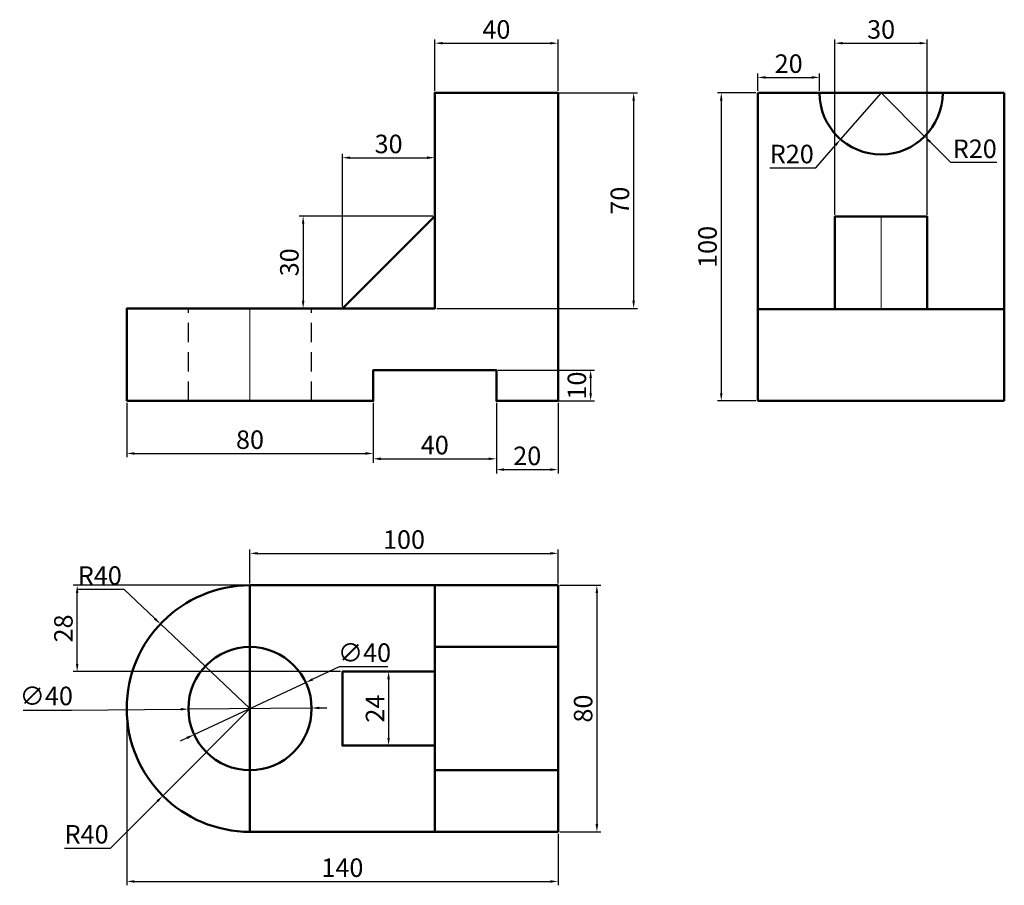
# Model space of a CAD drawing. Units: millimetres. Extents: x 40 to 360, y 50 to 331.
import ezdxf

# ---------------------------------------------------------------- set-up
doc = ezdxf.new("R2010")
doc.units = ezdxf.units.MM
doc.linetypes.add('CENTER', pattern=[50.8, 31.75, -6.35, 6.35, -6.35])
doc.linetypes.add('HIDDEN', pattern=[9.525, 6.35, -3.175])
for name, color, linetype, lineweight in [('M-CNTR', 4, 'CENTER', 18), ('M-DIMS', 2, 'Continuous', 25), ('M-HIDN', 3, 'HIDDEN', 25), ('M-OUTL', 7, 'Continuous', 50)]:
    doc.layers.add(name, color=color, linetype=linetype, lineweight=lineweight)
doc.styles.get("Standard").update_dxf_attribs({"font": 'arial.ttf'})
doc.dimstyles.new('ISO-25', dxfattribs={"dimtxt": 6, "dimasz": 2.5, "dimexe": 1.25, "dimexo": 0.625, "dimtad": 1, "dimtoh": 1, "dimdec": 0, "dimtxsty": 'Standard', "dimcen": 2.5, "dimadec": 0, "dimazin": 0, "dimtfac": 1, "dimtdec": 0, "dimtmove": 0, "dimatfit": 3, "dimfxl": 1, "dimarcsym": 0})

# ---------------------------------------------------------------- blocks, each defined once
blk = doc.blocks.new('*D1')
at = {"layer": 'Defpoints', "color": 0, "transparency": 16777216}
for p in [(74.87, 207.67), (154.87, 207.67), (154.87, 190.64)]:
    blk.add_point(p, dxfattribs=at)
at = {"layer": 'M-DIMS', "color": 0, "lineweight": -2, "transparency": 16777216}
for p, q in [((74.87, 207.05), (74.87, 189.39)), ((154.87, 207.05), (154.87, 189.39)), ((77.37, 190.64), (152.37, 190.64))]:
    blk.add_line(p, q, dxfattribs=at)
at = {"layer": 'M-DIMS', "color": 0, "transparency": 16777216}
for points in [[(77.37, 191.06), (77.37, 190.22), (74.87, 190.64)], [(152.37, 191.06), (152.37, 190.22), (154.87, 190.64)]]:
    blk.add_solid(points, dxfattribs=at)
at = {"layer": 'M-DIMS', "color": 0, "transparency": 16777216, "insert": (114.87, 194.33), "char_height": 6, "attachment_point": 5}
blk.add_mtext('80', dxfattribs=at)
blk = doc.blocks.new('*D2')
at = {"layer": 'Defpoints', "color": 0, "transparency": 16777216}
for p in [(154.87, 207.67), (194.87, 207.67), (194.87, 188.89)]:
    blk.add_point(p, dxfattribs=at)
at = {"layer": 'M-DIMS', "color": 0, "lineweight": -2, "transparency": 16777216}
for p, q in [((154.87, 207.05), (154.87, 187.64)), ((194.87, 207.05), (194.87, 187.64)), ((157.37, 188.89), (192.37, 188.89))]:
    blk.add_line(p, q, dxfattribs=at)
at = {"layer": 'M-DIMS', "color": 0, "transparency": 16777216}
for points in [[(157.37, 189.31), (157.37, 188.47), (154.87, 188.89)], [(192.37, 189.31), (192.37, 188.47), (194.87, 188.89)]]:
    blk.add_solid(points, dxfattribs=at)
at = {"layer": 'M-DIMS', "color": 0, "transparency": 16777216, "insert": (174.87, 192.58), "char_height": 6, "attachment_point": 5}
blk.add_mtext('40', dxfattribs=at)
blk = doc.blocks.new('*D3')
at = {"layer": 'Defpoints', "color": 0, "transparency": 16777216}
for p in [(194.87, 207.67), (214.87, 207.67), (214.87, 185.39)]:
    blk.add_point(p, dxfattribs=at)
at = {"layer": 'M-DIMS', "color": 0, "lineweight": -2, "transparency": 16777216}
for p, q in [((194.87, 207.05), (194.87, 184.14)), ((214.87, 207.05), (214.87, 184.14)), ((197.37, 185.39), (212.37, 185.39))]:
    blk.add_line(p, q, dxfattribs=at)
at = {"layer": 'M-DIMS', "color": 0, "transparency": 16777216}
for points in [[(197.37, 185.81), (197.37, 184.98), (194.87, 185.39)], [(212.37, 185.81), (212.37, 184.98), (214.87, 185.39)]]:
    blk.add_solid(points, dxfattribs=at)
at = {"layer": 'M-DIMS', "color": 0, "transparency": 16777216, "insert": (204.87, 189.08), "char_height": 6, "attachment_point": 5}
blk.add_mtext('20', dxfattribs=at)
blk = doc.blocks.new('*D4')
at = {"layer": 'Defpoints', "color": 0, "transparency": 16777216}
for p in [(174.87, 267.67), (132.12, 237.67), (174.87, 237.67)]:
    blk.add_point(p, dxfattribs=at)
at = {"layer": 'M-DIMS', "color": 0, "lineweight": -2, "transparency": 16777216}
for p, q in [((174.24, 267.67), (130.87, 267.67)), ((132.12, 265.17), (132.12, 240.17)), ((174.24, 237.67), (130.87, 237.67))]:
    blk.add_line(p, q, dxfattribs=at)
at = {"layer": 'M-DIMS', "color": 0, "transparency": 16777216}
for points in [[(131.71, 265.17), (132.54, 265.17), (132.12, 267.67)], [(131.71, 240.17), (132.54, 240.17), (132.12, 237.67)]]:
    blk.add_solid(points, dxfattribs=at)
at = {"layer": 'M-DIMS', "color": 0, "transparency": 16777216, "insert": (128.43, 252.67), "char_height": 6, "attachment_point": 5, "rotation": 90}
blk.add_mtext('30', dxfattribs=at)
blk = doc.blocks.new('*D5')
at = {"layer": 'Defpoints', "color": 0, "transparency": 16777216}
for p in [(174.87, 286.61), (144.87, 237.67), (174.87, 237.67)]:
    blk.add_point(p, dxfattribs=at)
at = {"layer": 'M-DIMS', "color": 0, "lineweight": -2, "transparency": 16777216}
for p, q in [((144.87, 238.3), (144.87, 287.86)), ((174.87, 238.3), (174.87, 287.86)), ((147.37, 286.61), (172.37, 286.61))]:
    blk.add_line(p, q, dxfattribs=at)
at = {"layer": 'M-DIMS', "color": 0, "transparency": 16777216}
for points in [[(147.37, 287.03), (147.37, 286.2), (144.87, 286.61)], [(172.37, 287.03), (172.37, 286.2), (174.87, 286.61)]]:
    blk.add_solid(points, dxfattribs=at)
at = {"layer": 'M-DIMS', "color": 0, "transparency": 16777216, "insert": (159.87, 290.3), "char_height": 6, "attachment_point": 5}
blk.add_mtext('30', dxfattribs=at)
blk = doc.blocks.new('*D6')
at = {"layer": 'Defpoints', "color": 0, "transparency": 16777216}
for p in [(174.87, 307.67), (174.87, 237.67), (239.42, 237.67)]:
    blk.add_point(p, dxfattribs=at)
at = {"layer": 'M-DIMS', "color": 0, "lineweight": -2, "transparency": 16777216}
for p, q in [((175.49, 307.67), (240.67, 307.67)), ((239.42, 305.17), (239.42, 240.17)), ((175.49, 237.67), (240.67, 237.67))]:
    blk.add_line(p, q, dxfattribs=at)
at = {"layer": 'M-DIMS', "color": 0, "transparency": 16777216}
for points in [[(239, 305.17), (239.83, 305.17), (239.42, 307.67)], [(239, 240.17), (239.83, 240.17), (239.42, 237.67)]]:
    blk.add_solid(points, dxfattribs=at)
at = {"layer": 'M-DIMS', "color": 0, "transparency": 16777216, "insert": (235.73, 272.67), "char_height": 6, "attachment_point": 5, "rotation": 90}
blk.add_mtext('70', dxfattribs=at)
blk = doc.blocks.new('*D7')
at = {"layer": 'Defpoints', "color": 0, "transparency": 16777216}
for p in [(194.87, 217.67), (194.87, 207.67), (225.46, 207.67)]:
    blk.add_point(p, dxfattribs=at)
at = {"layer": 'M-DIMS', "color": 0, "lineweight": -2, "transparency": 16777216}
for p, q in [((195.49, 217.67), (226.71, 217.67)), ((225.46, 215.17), (225.46, 210.17)), ((195.49, 207.67), (226.71, 207.67))]:
    blk.add_line(p, q, dxfattribs=at)
at = {"layer": 'M-DIMS', "color": 0, "transparency": 16777216}
for points in [[(225.05, 215.17), (225.88, 215.17), (225.46, 217.67)], [(225.05, 210.17), (225.88, 210.17), (225.46, 207.67)]]:
    blk.add_solid(points, dxfattribs=at)
at = {"layer": 'M-DIMS', "color": 0, "transparency": 16777216, "insert": (221.77, 212.67), "char_height": 6, "attachment_point": 5, "rotation": 90}
blk.add_mtext('10', dxfattribs=at)
blk = doc.blocks.new('*D8')
at = {"layer": 'Defpoints', "color": 0, "transparency": 16777216}
for p in [(279.75, 307.67), (267.86, 207.67), (279.75, 207.67)]:
    blk.add_point(p, dxfattribs=at)
at = {"layer": 'M-DIMS', "color": 0, "lineweight": -2, "transparency": 16777216}
for p, q in [((279.13, 307.67), (266.61, 307.67)), ((267.86, 305.17), (267.86, 210.17)), ((279.13, 207.67), (266.61, 207.67))]:
    blk.add_line(p, q, dxfattribs=at)
at = {"layer": 'M-DIMS', "color": 0, "transparency": 16777216}
for points in [[(267.45, 305.17), (268.28, 305.17), (267.86, 307.67)], [(267.45, 210.17), (268.28, 210.17), (267.86, 207.67)]]:
    blk.add_solid(points, dxfattribs=at)
at = {"layer": 'M-DIMS', "color": 0, "transparency": 16777216, "insert": (264.18, 257.67), "char_height": 6, "attachment_point": 5, "rotation": 90}
blk.add_mtext('100', dxfattribs=at)
blk = doc.blocks.new('*D9')
at = {"layer": 'Defpoints', "color": 0, "transparency": 16777216}
for p in [(299.75, 312.67), (279.75, 307.67), (299.75, 307.67)]:
    blk.add_point(p, dxfattribs=at)
at = {"layer": 'M-DIMS', "color": 0, "lineweight": -2, "transparency": 16777216}
for p, q in [((279.75, 308.3), (279.75, 313.92)), ((299.75, 308.3), (299.75, 313.92)), ((282.25, 312.67), (297.25, 312.67))]:
    blk.add_line(p, q, dxfattribs=at)
at = {"layer": 'M-DIMS', "color": 0, "transparency": 16777216}
for points in [[(282.25, 313.09), (282.25, 312.26), (279.75, 312.67)], [(297.25, 313.09), (297.25, 312.26), (299.75, 312.67)]]:
    blk.add_solid(points, dxfattribs=at)
at = {"layer": 'M-DIMS', "color": 0, "transparency": 16777216, "insert": (289.75, 316.36), "char_height": 6, "attachment_point": 5}
blk.add_mtext('20', dxfattribs=at)
blk = doc.blocks.new('*D10')
at = {"layer": 'Defpoints', "color": 0, "transparency": 16777216}
for p in [(319.75, 307.67), (306.61, 292.59)]:
    blk.add_point(p, dxfattribs=at)
at = {"layer": 'M-DIMS', "color": 0, "lineweight": -2, "transparency": 16777216}
for p, q in [((319.75, 307.67), (306.61, 292.59)), ((298.55, 283.34), (304.97, 290.71)), ((283.61, 283.34), (298.55, 283.34))]:
    blk.add_line(p, q, dxfattribs=at)
at = {"layer": 'M-DIMS', "color": 0, "transparency": 16777216}
blk.add_solid([(304.66, 290.98), (305.28, 290.44), (306.61, 292.59)], dxfattribs=at)
at = {"layer": 'M-DIMS', "color": 0, "transparency": 16777216, "insert": (290.76, 287.03), "char_height": 6, "attachment_point": 5}
blk.add_mtext('R20', dxfattribs=at)
blk = doc.blocks.new('*D11')
at = {"layer": 'Defpoints', "color": 0, "transparency": 16777216}
for p in [(159.87, 119.84), (159.87, 95.84), (159.87, 95.84)]:
    blk.add_point(p, dxfattribs=at)
at = {"layer": 'M-DIMS', "color": 0, "lineweight": -2, "transparency": 16777216}
for p, q in [((160.49, 119.84), (161.12, 119.84)), ((159.87, 117.34), (159.87, 98.34)), ((160.49, 95.84), (161.12, 95.84))]:
    blk.add_line(p, q, dxfattribs=at)
at = {"layer": 'M-DIMS', "color": 0, "transparency": 16777216}
for points in [[(159.45, 117.34), (160.28, 117.34), (159.87, 119.84)], [(159.45, 98.34), (160.28, 98.34), (159.87, 95.84)]]:
    blk.add_solid(points, dxfattribs=at)
at = {"layer": 'M-DIMS', "color": 0, "transparency": 16777216, "insert": (156.23, 107.84), "char_height": 6, "attachment_point": 5, "rotation": 90}
blk.add_mtext('24', dxfattribs=at)
blk = doc.blocks.new('*D12')
at = {"layer": 'Defpoints', "color": 0, "transparency": 16777216}
for p in [(94.87, 107.65), (134.86, 108.02)]:
    blk.add_point(p, dxfattribs=at)
at = {"layer": 'M-DIMS', "color": 0, "lineweight": -2, "transparency": 16777216}
for p, q in [((41.19, 107.3), (56.92, 107.3)), ((56.92, 107.3), (92.37, 107.63)), ((134.86, 108.02), (94.87, 107.65)), ((137.36, 108.05), (139.86, 108.07))]:
    blk.add_line(p, q, dxfattribs=at)
at = {"layer": 'M-DIMS', "color": 0, "transparency": 16777216}
for points in [[(92.36, 108.05), (92.37, 107.21), (94.87, 107.65)], [(137.36, 108.46), (137.37, 107.63), (134.86, 108.02)]]:
    blk.add_solid(points, dxfattribs=at)
at = {"layer": 'M-DIMS', "color": 0, "transparency": 16777216, "insert": (48.75, 111.16), "char_height": 6, "attachment_point": 5}
blk.add_mtext('∅40', dxfattribs=at)
blk = doc.blocks.new('*D13')
at = {"layer": 'Defpoints', "color": 0, "transparency": 16777216}
for p in [(85.8, 135.31), (114.87, 107.84)]:
    blk.add_point(p, dxfattribs=at)
at = {"layer": 'M-DIMS', "color": 0, "lineweight": -2, "transparency": 16777216}
for p, q in [((58.97, 146.55), (73.91, 146.55)), ((73.91, 146.55), (83.98, 137.03)), ((114.87, 107.84), (85.8, 135.31))]:
    blk.add_line(p, q, dxfattribs=at)
at = {"layer": 'M-DIMS', "color": 0, "transparency": 16777216}
blk.add_solid([(84.26, 137.34), (83.69, 136.73), (85.8, 135.31)], dxfattribs=at)
at = {"layer": 'M-DIMS', "color": 0, "transparency": 16777216, "insert": (66.12, 150.24), "char_height": 6, "attachment_point": 5}
blk.add_mtext('R40', dxfattribs=at)
blk = doc.blocks.new('*D14')
at = {"layer": 'Defpoints', "color": 0, "transparency": 16777216}
for p in [(214.87, 158.22), (114.87, 147.84), (214.87, 147.84)]:
    blk.add_point(p, dxfattribs=at)
at = {"layer": 'M-DIMS', "color": 0, "lineweight": -2, "transparency": 16777216}
for p, q in [((114.87, 148.46), (114.87, 159.47)), ((117.37, 158.22), (212.37, 158.22)), ((214.87, 148.46), (214.87, 159.47))]:
    blk.add_line(p, q, dxfattribs=at)
at = {"layer": 'M-DIMS', "color": 0, "transparency": 16777216}
for points in [[(117.37, 158.64), (117.37, 157.8), (114.87, 158.22)], [(212.37, 158.64), (212.37, 157.8), (214.87, 158.22)]]:
    blk.add_solid(points, dxfattribs=at)
at = {"layer": 'M-DIMS', "color": 0, "transparency": 16777216, "insert": (164.87, 161.91), "char_height": 6, "attachment_point": 5}
blk.add_mtext('100', dxfattribs=at)
blk = doc.blocks.new('*D15')
at = {"layer": 'Defpoints', "color": 0, "transparency": 16777216}
for p in [(214.87, 147.84), (214.87, 67.84), (227.49, 67.84)]:
    blk.add_point(p, dxfattribs=at)
at = {"layer": 'M-DIMS', "color": 0, "lineweight": -2, "transparency": 16777216}
for p, q in [((215.49, 147.84), (228.74, 147.84)), ((227.49, 145.34), (227.49, 70.34)), ((215.49, 67.84), (228.74, 67.84))]:
    blk.add_line(p, q, dxfattribs=at)
at = {"layer": 'M-DIMS', "color": 0, "transparency": 16777216}
for points in [[(227.07, 145.34), (227.91, 145.34), (227.49, 147.84)], [(227.07, 70.34), (227.91, 70.34), (227.49, 67.84)]]:
    blk.add_solid(points, dxfattribs=at)
at = {"layer": 'M-DIMS', "color": 0, "transparency": 16777216, "insert": (223.8, 107.84), "char_height": 6, "attachment_point": 5, "rotation": 90}
blk.add_mtext('80', dxfattribs=at)
blk = doc.blocks.new('*D16')
at = {"layer": 'Defpoints', "color": 0, "transparency": 16777216}
for p in [(74.87, 107.84), (214.87, 67.84), (214.87, 51.74)]:
    blk.add_point(p, dxfattribs=at)
at = {"layer": 'M-DIMS', "color": 0, "lineweight": -2, "transparency": 16777216}
for p, q in [((74.87, 107.21), (74.87, 50.49)), ((214.87, 67.21), (214.87, 50.49)), ((77.37, 51.74), (212.37, 51.74))]:
    blk.add_line(p, q, dxfattribs=at)
at = {"layer": 'M-DIMS', "color": 0, "transparency": 16777216}
for points in [[(77.37, 52.16), (77.37, 51.32), (74.87, 51.74)], [(212.37, 52.16), (212.37, 51.32), (214.87, 51.74)]]:
    blk.add_solid(points, dxfattribs=at)
at = {"layer": 'M-DIMS', "color": 0, "transparency": 16777216, "insert": (144.87, 55.43), "char_height": 6, "attachment_point": 5}
blk.add_mtext('140', dxfattribs=at)
blk = doc.blocks.new('*D17')
at = {"layer": 'Defpoints', "color": 0, "transparency": 16777216}
for p in [(214.87, 323.77), (174.87, 307.67), (214.87, 307.67)]:
    blk.add_point(p, dxfattribs=at)
at = {"layer": 'M-DIMS', "color": 0, "lineweight": -2, "transparency": 16777216}
for p, q in [((174.87, 308.3), (174.87, 325.02)), ((177.37, 323.77), (212.37, 323.77)), ((214.87, 308.3), (214.87, 325.02))]:
    blk.add_line(p, q, dxfattribs=at)
at = {"layer": 'M-DIMS', "color": 0, "transparency": 16777216}
for points in [[(177.37, 324.19), (177.37, 323.36), (174.87, 323.77)], [(212.37, 324.19), (212.37, 323.36), (214.87, 323.77)]]:
    blk.add_solid(points, dxfattribs=at)
at = {"layer": 'M-DIMS', "color": 0, "transparency": 16777216, "insert": (194.87, 327.46), "char_height": 6, "attachment_point": 5}
blk.add_mtext('40', dxfattribs=at)
blk = doc.blocks.new('*D18')
at = {"layer": 'Defpoints', "color": 0, "transparency": 16777216}
for p in [(58.77, 147.84), (174.87, 147.84), (144.87, 119.84)]:
    blk.add_point(p, dxfattribs=at)
at = {"layer": 'M-DIMS', "color": 0, "lineweight": -2, "transparency": 16777216}
for p, q in [((174.24, 147.84), (57.52, 147.84)), ((58.77, 122.34), (58.77, 145.34)), ((144.24, 119.84), (57.52, 119.84))]:
    blk.add_line(p, q, dxfattribs=at)
at = {"layer": 'M-DIMS', "color": 0, "transparency": 16777216}
for points in [[(58.35, 145.34), (59.18, 145.34), (58.77, 147.84)], [(58.35, 122.34), (59.18, 122.34), (58.77, 119.84)]]:
    blk.add_solid(points, dxfattribs=at)
at = {"layer": 'M-DIMS', "color": 0, "transparency": 16777216, "insert": (55.08, 133.84), "char_height": 6, "attachment_point": 5, "rotation": 90}
blk.add_mtext('28', dxfattribs=at)
blk = doc.blocks.new('*D19')
at = {"layer": 'Defpoints', "color": 0, "transparency": 16777216}
for p in [(334.75, 323.77), (304.75, 267.48), (334.75, 267.48)]:
    blk.add_point(p, dxfattribs=at)
at = {"layer": 'M-DIMS', "color": 0, "lineweight": -2, "transparency": 16777216}
for p, q in [((304.75, 268.1), (304.75, 325.02)), ((307.25, 323.77), (332.25, 323.77)), ((334.75, 268.1), (334.75, 325.02))]:
    blk.add_line(p, q, dxfattribs=at)
at = {"layer": 'M-DIMS', "color": 0, "transparency": 16777216}
for points in [[(307.25, 324.19), (307.25, 323.36), (304.75, 323.77)], [(332.25, 324.19), (332.25, 323.36), (334.75, 323.77)]]:
    blk.add_solid(points, dxfattribs=at)
at = {"layer": 'M-DIMS', "color": 0, "transparency": 16777216, "insert": (319.75, 327.46), "char_height": 6, "attachment_point": 5}
blk.add_mtext('30', dxfattribs=at)
blk = doc.blocks.new('*D20')
at = {"layer": 'Defpoints', "color": 0, "transparency": 16777216}
for p in [(114.87, 107.84), (86.58, 79.55)]:
    blk.add_point(p, dxfattribs=at)
at = {"layer": 'M-DIMS', "color": 0, "lineweight": -2, "transparency": 16777216}
for p, q in [((114.87, 107.84), (86.58, 79.55)), ((69.61, 62.58), (84.82, 77.78)), ((54.67, 62.58), (69.61, 62.58))]:
    blk.add_line(p, q, dxfattribs=at)
at = {"layer": 'M-DIMS', "color": 0, "transparency": 16777216}
blk.add_solid([(84.52, 78.08), (85.11, 77.49), (86.58, 79.55)], dxfattribs=at)
at = {"layer": 'M-DIMS', "color": 0, "transparency": 16777216, "insert": (61.83, 66.27), "char_height": 6, "attachment_point": 5}
blk.add_mtext('R40', dxfattribs=at)
blk = doc.blocks.new('*D21')
at = {"layer": 'Defpoints', "color": 0, "transparency": 16777216}
for p in [(132.99, 116.29), (96.74, 99.39)]:
    blk.add_point(p, dxfattribs=at)
at = {"layer": 'M-DIMS', "color": 0, "lineweight": -2, "transparency": 16777216}
for p, q in [((143.87, 121.36), (135.26, 117.35)), ((159.59, 121.36), (143.87, 121.36)), ((96.74, 99.39), (132.99, 116.29)), ((94.47, 98.33), (92.21, 97.27))]:
    blk.add_line(p, q, dxfattribs=at)
at = {"layer": 'M-DIMS', "color": 0, "transparency": 16777216}
for points in [[(135.08, 117.72), (135.43, 116.97), (132.99, 116.29)], [(94.3, 98.71), (94.65, 97.95), (96.74, 99.39)]]:
    blk.add_solid(points, dxfattribs=at)
at = {"layer": 'M-DIMS', "color": 0, "transparency": 16777216, "insert": (152.04, 125.22), "char_height": 6, "attachment_point": 5}
blk.add_mtext('∅40', dxfattribs=at)
blk = doc.blocks.new('*D22')
at = {"layer": 'Defpoints', "color": 0, "transparency": 16777216}
for p in [(319.75, 307.67), (333.89, 293.53)]:
    blk.add_point(p, dxfattribs=at)
at = {"layer": 'M-DIMS', "color": 0, "lineweight": -2, "transparency": 16777216}
for p, q in [((319.75, 307.67), (333.89, 293.53)), ((342.38, 285.04), (335.66, 291.76)), ((357.32, 285.04), (342.38, 285.04))]:
    blk.add_line(p, q, dxfattribs=at)
at = {"layer": 'M-DIMS', "color": 0, "transparency": 16777216}
blk.add_solid([(335.95, 292.05), (335.36, 291.47), (333.89, 293.53)], dxfattribs=at)
at = {"layer": 'M-DIMS', "color": 0, "transparency": 16777216, "insert": (350.16, 288.73), "char_height": 6, "attachment_point": 5}
blk.add_mtext('R20', dxfattribs=at)

msp = doc.modelspace()

# ---------------------------------------------------------------- linework, layer by layer
at = {"layer": 'M-CNTR'}
for p, q in [((319.75, 237.48), (319.75, 267.48)), ((114.87, 207.67), (114.87, 237.67))]:
    msp.add_line(p, q, dxfattribs=at)
at = {"layer": 'M-HIDN'}
for p, q in [((94.87, 207.67), (94.87, 237.67)), ((134.87, 207.67), (134.87, 237.67))]:
    msp.add_line(p, q, dxfattribs=at)
at = {"layer": 'M-OUTL'}
for p, q in [((279.75, 307.67), (279.75, 207.67)), ((279.75, 307.67), (299.75, 307.67)), ((359.75, 307.67), (339.75, 307.67)), ((359.75, 207.67), (359.75, 307.67)), ((174.87, 267.67), (144.87, 237.67)), ((279.75, 237.48), (359.75, 237.48)), ((279.75, 207.67), (359.75, 207.67)), ((114.87, 147.84), (214.87, 147.84)), ((174.87, 147.84), (174.87, 67.84)), ((214.87, 147.84), (214.87, 67.84)), ((174.87, 127.84), (214.87, 127.84)), ((174.87, 87.84), (214.87, 87.84)), ((214.87, 67.84), (114.87, 67.84))]:
    msp.add_line(p, q, dxfattribs=at)
msp.add_lwpolyline([(74.87, 207.67), (154.87, 207.67), (154.87, 217.67), (194.87, 217.67), (194.87, 207.67), (214.87, 207.67), (214.87, 307.67), (174.87, 307.67), (174.87, 237.67), (74.87, 237.67)], close=True, dxfattribs=at)
for points in [[(299.75, 307.67, 1), (339.75, 307.67)], [(114.87, 147.84, 1), (114.87, 67.84)]]:
    msp.add_lwpolyline(points, format="xyb", close=True, dxfattribs=at)
for points in [[(304.75, 237.48), (304.75, 267.48), (334.75, 267.48), (334.75, 237.48)], [(174.87, 119.84), (144.87, 119.84), (144.87, 95.84), (174.87, 95.84)]]:
    msp.add_lwpolyline(points, dxfattribs=at)
msp.add_circle((114.87, 107.84), 20, dxfattribs=at)

# ---------------------------------------------------------------- dimensions: what is measured, and where the dimension line sits
at = {"layer": 'M-DIMS'}
for base, p1, p2, override, picture, middle in [((214.87, 323.77), (174.87, 307.67), (214.87, 307.67), {"dimdec": 0, "dimlfac": 1, "dimrnd": 0, "dimzin": 0, "dimdsep": 46, "dimlunit": 2}, '*D17', (194.87, 327.46)), ((334.75, 323.77), (304.75, 267.48), (334.75, 267.48), {"dimdec": 0, "dimlfac": 1, "dimrnd": 0, "dimzin": 0, "dimdsep": 46, "dimlunit": 2}, '*D19', (319.75, 327.46)), ((299.75, 312.67), (279.75, 307.67), (299.75, 307.67), {"dimclrd": 0, "dimclre": 0, "dimclrt": 0}, '*D9', (289.75, 316.36)), ((174.87, 286.61), (144.87, 237.67), (174.87, 237.67), {"dimclrd": 0, "dimclre": 0, "dimclrt": 0}, '*D5', (159.87, 290.3)), ((154.87, 190.64), (74.87, 207.67), (154.87, 207.67), {"dimclrd": 0, "dimclre": 0, "dimclrt": 0}, '*D1', (114.87, 194.33)), ((194.87, 188.89), (154.87, 207.67), (194.87, 207.67), {"dimclrd": 0, "dimclre": 0, "dimclrt": 0}, '*D2', (174.87, 192.58)), ((214.87, 185.39), (194.87, 207.67), (214.87, 207.67), {"dimclrd": 0, "dimclre": 0, "dimclrt": 0}, '*D3', (204.87, 189.08)), ((214.87, 158.22), (114.87, 147.84), (214.87, 147.84), {"dimclrd": 0, "dimclre": 0, "dimclrt": 0}, '*D14', (164.87, 161.91)), ((214.87, 51.74), (74.87, 107.84), (214.87, 67.84), {"dimdec": 0, "dimlfac": 1, "dimrnd": 0, "dimzin": 0, "dimdsep": 46, "dimlunit": 2}, '*D16', (144.87, 55.43))]:
    dim = msp.add_linear_dim(base=base, p1=p1, p2=p2, dimstyle='ISO-25', override=override, dxfattribs=at)
    dim.commit()
    dim.dimension.update_dxf_attribs({"geometry": picture, "text_midpoint": middle})
for base, p1, p2, override, picture, middle in [((239.42, 237.67), (174.87, 307.67), (174.87, 237.67), {"dimclrd": 0, "dimclre": 0, "dimclrt": 0}, '*D6', (235.73, 272.67)), ((267.86, 207.67), (279.75, 307.67), (279.75, 207.67), {"dimclrd": 0, "dimclre": 0, "dimclrt": 0}, '*D8', (264.18, 257.67)), ((132.12, 237.67), (174.87, 267.67), (174.87, 237.67), {"dimclrd": 0, "dimclre": 0, "dimclrt": 0}, '*D4', (128.43, 252.67)), ((225.46, 207.67), (194.87, 217.67), (194.87, 207.67), {"dimclrd": 0, "dimclre": 0, "dimclrt": 0}, '*D7', (221.77, 212.67)), ((58.77, 147.84), (144.87, 119.84), (174.87, 147.84), {"dimdec": 0, "dimlfac": 1, "dimrnd": 0, "dimzin": 0, "dimdsep": 46, "dimlunit": 2}, '*D18', (55.08, 133.84)), ((227.49, 67.84), (214.87, 147.84), (214.87, 67.84), {"dimclrd": 0, "dimclre": 0, "dimclrt": 0}, '*D15', (223.8, 107.84)), ((159.87, 95.84), (159.87, 119.84), (159.87, 95.84), {"dimclrd": 0, "dimclre": 0, "dimclrt": 0}, '*D11', (156.23, 107.84))]:
    dim = msp.add_linear_dim(base=base, p1=p1, p2=p2, angle=90, dimstyle='ISO-25', override=override, dxfattribs=at)
    dim.commit()
    dim.dimension.update_dxf_attribs({"geometry": picture, "text_midpoint": middle})
for center, mpoint, override, picture, middle in [((319.75, 307.67), (306.61, 292.59), {"dimclrd": 0, "dimclre": 0, "dimclrt": 0}, '*D10', (290.76, 283.34)), ((319.75, 307.67), (333.89, 293.53), {"dimdec": 0, "dimlfac": 1, "dimrnd": 0, "dimzin": 0, "dimdsep": 46, "dimlunit": 2}, '*D22', (350.16, 285.04)), ((114.87, 107.84), (85.8, 135.31), {"dimclrd": 0, "dimclre": 0, "dimclrt": 0}, '*D13', (66.12, 146.55)), ((114.87, 107.84), (86.58, 79.55), {"dimdec": 0, "dimlfac": 1, "dimrnd": 0, "dimzin": 0, "dimdsep": 46, "dimlunit": 2}, '*D20', (61.83, 62.58))]:
    dim = msp.add_radius_dim(center=center, mpoint=mpoint, dimstyle='ISO-25', override=override, dxfattribs=at)
    dim.commit()
    dim.dimension.update_dxf_attribs({"geometry": picture, "text_midpoint": middle, "dimtype": 164})
for p1, p2, override, picture, middle in [((96.74, 99.39), (132.99, 116.29), {"dimdec": 0, "dimlfac": 1, "dimrnd": 0, "dimzin": 0, "dimdsep": 46, "dimlunit": 2}, '*D21', (152.04, 121.36)), ((134.86, 108.02), (94.87, 107.65), {"dimclrd": 0, "dimclre": 0, "dimclrt": 0}, '*D12', (56.92, 107.3))]:
    dim = msp.add_diameter_dim_2p(p1=p1, p2=p2, dimstyle='ISO-25', override=override, dxfattribs=at)
    dim.commit()
    dim.dimension.update_dxf_attribs({"geometry": picture, "text_midpoint": middle, "dimtype": 163})

doc.saveas('drawing.dxf')
